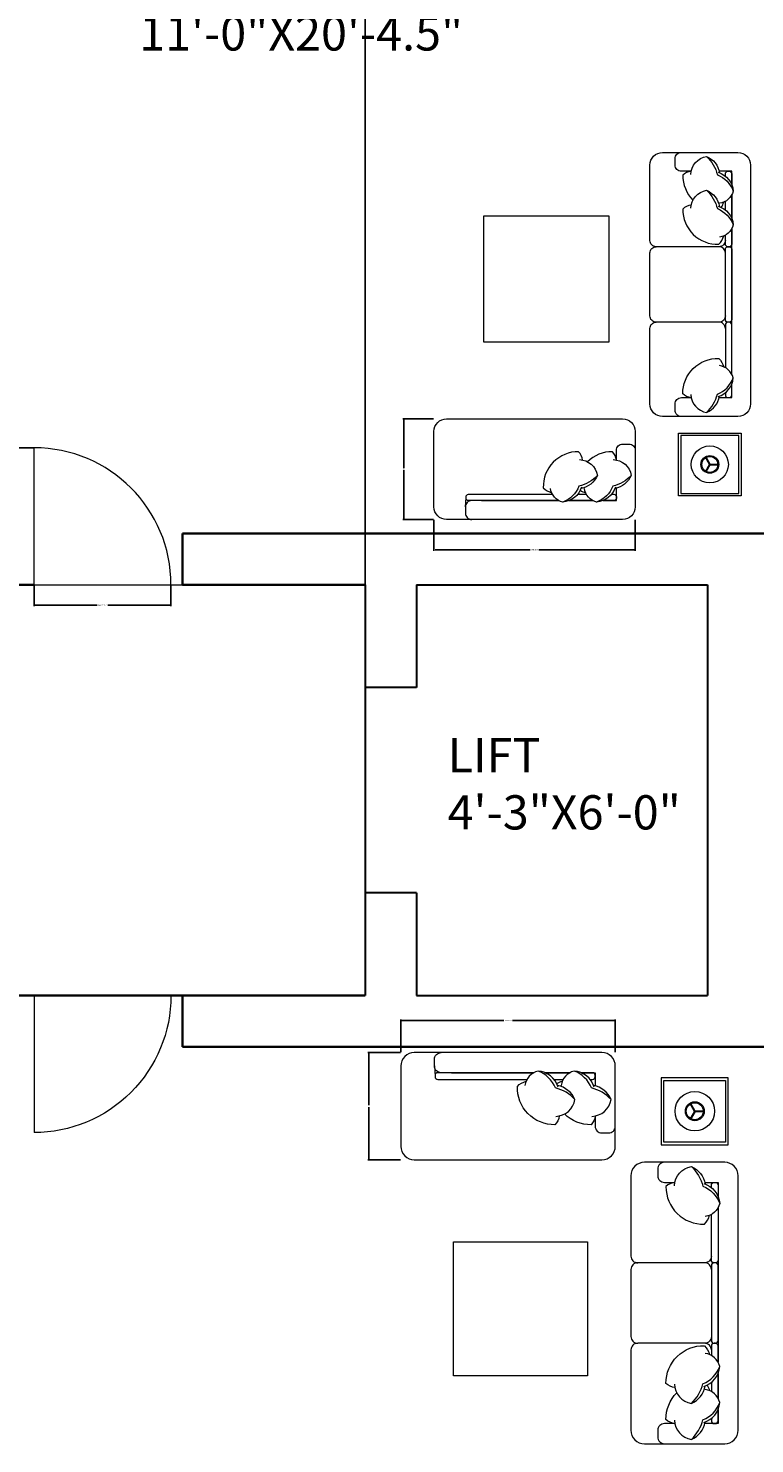
# Model space of a CAD drawing. Units: inches. Extents: x -59 to 444, y -680 to 63.
# Tile 6 of 9: x 132 to 260, y -423 to -175. Entities that reach past the tile are written whole.
import ezdxf

# ---------------------------------------------------------------- set-up
doc = ezdxf.new("R2010")
doc.units = ezdxf.units.IN
doc.header["$MEASUREMENT"] = 0
for name, color, linetype, lineweight in [('A-ANNO-DIMS', 2, 'Continuous', 18), ('A-AREA-IDEN', 7, 'Continuous', 18), ('A-DOOR', 3, 'Continuous', 18), ('A-FLOR-EVTR', 7, 'Continuous', 30), ('A-FURN', 8, 'Continuous', 13), ('A-WALL', 7, 'Continuous', 35)]:
    doc.layers.add(name, color=color, linetype=linetype, lineweight=lineweight)
doc.styles.get("Standard").update_dxf_attribs({"font": 'arial.ttf'})
doc.dimstyles.get("Standard").update_dxf_attribs({"dimtxt": 0.18, "dimasz": 0.18, "dimexe": 0.18, "dimexo": 0.0625, "dimgap": 0.09, "dimtad": 0, "dimtih": 1, "dimtoh": 1, "dimdec": 0, "dimzin": 0, "dimdsep": 46, "dimlunit": 3, "dimtxsty": 'Standard', "dimcen": 0.09, "dimadec": 0, "dimazin": 0, "dimtfac": 1, "dimtdec": 0, "dimtofl": 0, "dimtmove": 0, "dimatfit": 3, "dimfxl": 1, "dimtolj": 1, "dimtzin": 0, "dimarcsym": 0})

# ---------------------------------------------------------------- blocks, each defined once
blk = doc.blocks.new('DAY BED1')
at = {"color": 0}
blk.add_line((0.3, 0.25), (0.225, 0.255), dxfattribs=at)
blk.add_lwpolyline([(-0.3, 0, -0.414214), (-0.4, 0.1), (-0.4, 0.1, 0.317837), (-0.4, 0.1, -0.414214), (-0.4, 0.1), (-0.4, 0.1, 1.186185), (-0.4, 0.1, -0.414214), (-0.4, 0.1), (-0.4, 1.5, -0.414214), (-0.3, 1.6), (0.3, 1.6, -0.414214), (0.4, 1.5), (0.4, 0.1, -0.414214), (0.3, 0)], format="xyb", close=True, dxfattribs=at)
for points in [[(-0.073, 1.45), (-0.15, 1.45, -0.414214), (-0.2, 1.5), (-0.2, 1.55, -0.414214), (-0.15, 1.6)], [(-0.076, 1.425, -0.356772), (0.05, 1.568, -0.249542), (0.154, 1.438, 9.61688)], [(0.05, 1.568, -0.14773), (0.136, 1.422, -0.213343), (0.262, 1.293, -0.178662)], [(-0.073, 1.45, 0.165541), (-0.139, 1.419, 0.200231), (-0.058, 1.221, 0.121523)], [(0.143, 1.442, -0.306663), (0.262, 1.293, -0.30633), (0.154, 1.196, 0.872847)], [(0.25, 1.345), (0.25, 1.45), (0.152, 1.45, -0.414214)], [(0.2, 1.412), (0.2, 1.43, -0.414214), (0.22, 1.45), (0.23, 1.45, -0.414214), (0.25, 1.43)], [(0.25, 1.43), (0.25, 1.345, -0.414214)], [(-0.076, 1.156, -0.356772), (0.05, 1.299, -0.249542), (0.154, 1.169, 9.61688)], [(0.05, 1.299, -0.14773), (0.136, 1.153, -0.213343), (0.262, 1.024, -0.178662)], [(-0.073, 1.181, 0.165541), (-0.139, 1.15, 0.425989), (0.148, 0.869, 0.121523), (0.187, 0.936, -7.115464)], [(0.143, 1.173, -0.306663), (0.262, 1.024, -0.30633), (0.154, 0.926, 0.872847)], [(0.168, 1.163, 0.071865), (0.187, 1.205, -7.115464)], [(0.2, 1.142), (0.2, 1.211, -0.414214)], [(0.25, 1.262), (0.25, 1.075, -0.414214)], [(0.25, 0.992), (0.25, 0.275, -0.414214), (0.23, 0.255), (0.22, 0.255, -0.414214), (0.2, 0.275), (0.2, 0.942, -0.414214)], [(0.25, 0.377), (0.25, 0.3, 0.414214), (0.3, 0.25), (0.35, 0.25, 0.414214), (0.4, 0.3)]]:
    blk.add_lwpolyline(points, format="xyb", dxfattribs=at)
for points in [[(0.25, 1.075), (0.25, 1.262)], [(0.25, 0.377), (0.25, 0.992)]]:
    blk.add_lwpolyline(points, dxfattribs=at)
blk = doc.blocks.new('DOOR-SWING-24')
blk.add_line((24, 0), (0, 0))
blk.add_arc((24, 0), 24, 90, 180)
blk = doc.blocks.new('*D16')
at = {"layer": 'A-ANNO-DIMS', "color": 0, "lineweight": -2, "transparency": 16777216}
for p, q in [((133.23, -272.5), (133.23, -276.22)), ((157.23, -272.5), (157.23, -276.22)), ((133.41, -276.04), (144.29, -276.04)), ((157.05, -276.04), (146.17, -276.04))]:
    blk.add_line(p, q, dxfattribs=at)
at = {"layer": 'A-ANNO-DIMS', "color": 0, "transparency": 16777216}
for points in [[(133.41, -276.01), (133.41, -276.07), (133.23, -276.04)], [(157.05, -276.01), (157.05, -276.07), (157.23, -276.04)]]:
    blk.add_solid(points, dxfattribs=at)
at = {"layer": 'Defpoints', "color": 0, "transparency": 16777216}
for p in [(133.23, -272.44), (157.23, -272.44), (157.23, -276.04)]:
    blk.add_point(p, dxfattribs=at)
at = {"layer": 'A-ANNO-DIMS', "color": 0, "transparency": 16777216, "insert": (145.23, -276.04), "char_height": 0.18, "attachment_point": 5}
blk.add_mtext('\\A1;DOOR 24 TYP.', dxfattribs=at)
blk = doc.blocks.new('*D17')
at = {"layer": 'A-ANNO-DIMS', "color": 0, "lineweight": -2, "transparency": 16777216}
for p, q in [((133.17, -248.44), (129.45, -248.44)), ((129.63, -248.62), (129.63, -260.25)), ((129.63, -272.26), (129.63, -260.62)), ((133.17, -272.44), (129.45, -272.44))]:
    blk.add_line(p, q, dxfattribs=at)
at = {"layer": 'A-ANNO-DIMS', "color": 0, "transparency": 16777216}
for points in [[(129.6, -248.62), (129.66, -248.62), (129.63, -248.44)], [(129.6, -272.26), (129.66, -272.26), (129.63, -272.44)]]:
    blk.add_solid(points, dxfattribs=at)
at = {"layer": 'Defpoints', "color": 0, "transparency": 16777216}
for p in [(133.23, -248.44), (129.63, -272.44), (133.23, -272.44)]:
    blk.add_point(p, dxfattribs=at)
at = {"layer": 'A-ANNO-DIMS', "color": 0, "transparency": 16777216, "insert": (129.63, -260.44), "char_height": 0.18, "attachment_point": 5}
blk.add_mtext('\\A1;24 TYP.', dxfattribs=at)
blk = doc.blocks.new('*D42')
at = {"layer": 'A-ANNO-DIMS', "color": 0, "lineweight": -2, "transparency": 16777216}
for p, q in [((203.31, -261.07), (203.31, -266.48)), ((238.57, -261.07), (238.57, -266.48)), ((203.49, -266.3), (220.17, -266.3)), ((238.39, -266.3), (221.7, -266.3))]:
    blk.add_line(p, q, dxfattribs=at)
at = {"layer": 'A-ANNO-DIMS', "color": 0, "transparency": 16777216}
for points in [[(203.49, -266.27), (203.49, -266.33), (203.31, -266.3)], [(238.39, -266.27), (238.39, -266.33), (238.57, -266.3)]]:
    blk.add_solid(points, dxfattribs=at)
at = {"layer": 'Defpoints', "color": 0, "transparency": 16777216}
for p in [(203.31, -261.01), (238.57, -261.01), (238.57, -266.3)]:
    blk.add_point(p, dxfattribs=at)
at = {"layer": 'A-ANNO-DIMS', "color": 0, "transparency": 16777216, "insert": (220.94, -266.3), "char_height": 0.18, "attachment_point": 5}
blk.add_mtext('\\A1;DAYBED 35', dxfattribs=at)
blk = doc.blocks.new('*D43')
at = {"layer": 'A-ANNO-DIMS', "color": 0, "lineweight": -2, "transparency": 16777216}
for p, q in [((203.25, -243.38), (197.84, -243.38)), ((198.02, -243.56), (198.02, -252.01)), ((198.02, -260.83), (198.02, -252.38)), ((203.25, -261.01), (197.84, -261.01))]:
    blk.add_line(p, q, dxfattribs=at)
at = {"layer": 'A-ANNO-DIMS', "color": 0, "transparency": 16777216}
for points in [[(197.99, -243.56), (198.05, -243.56), (198.02, -243.38)], [(197.99, -260.83), (198.05, -260.83), (198.02, -261.01)]]:
    blk.add_solid(points, dxfattribs=at)
at = {"layer": 'Defpoints', "color": 0, "transparency": 16777216}
for p in [(203.31, -243.38), (198.02, -261.01), (203.31, -261.01)]:
    blk.add_point(p, dxfattribs=at)
at = {"layer": 'A-ANNO-DIMS', "color": 0, "transparency": 16777216, "insert": (198.02, -252.19), "char_height": 0.18, "attachment_point": 5}
blk.add_mtext('\\A1;18', dxfattribs=at)
blk = doc.blocks.new('*D44')
at = {"layer": 'A-ANNO-DIMS', "color": 0, "lineweight": -2, "transparency": 16777216}
for p, q in [((197.51, -354.37), (197.51, -348.62)), ((197.69, -348.8), (215.53, -348.8)), ((234.9, -348.8), (217.06, -348.8)), ((235.08, -354.37), (235.08, -348.62))]:
    blk.add_line(p, q, dxfattribs=at)
at = {"layer": 'A-ANNO-DIMS', "color": 0, "transparency": 16777216}
for points in [[(197.69, -348.77), (197.69, -348.83), (197.51, -348.8)], [(234.9, -348.77), (234.9, -348.83), (235.08, -348.8)]]:
    blk.add_solid(points, dxfattribs=at)
at = {"layer": 'Defpoints', "color": 0, "transparency": 16777216}
for p in [(235.08, -348.8), (197.51, -354.43), (235.08, -354.43)]:
    blk.add_point(p, dxfattribs=at)
at = {"layer": 'A-ANNO-DIMS', "color": 0, "transparency": 16777216, "insert": (216.29, -348.8), "char_height": 0.18, "attachment_point": 5}
blk.add_mtext('\\A1;DAYBED 38', dxfattribs=at)
blk = doc.blocks.new('*D45')
at = {"layer": 'A-ANNO-DIMS', "color": 0, "lineweight": -2, "transparency": 16777216}
for p, q in [((197.45, -354.43), (191.7, -354.43)), ((191.88, -354.61), (191.88, -363.64)), ((191.88, -373.03), (191.88, -364)), ((197.45, -373.21), (191.7, -373.21))]:
    blk.add_line(p, q, dxfattribs=at)
at = {"layer": 'A-ANNO-DIMS', "color": 0, "transparency": 16777216}
for points in [[(191.85, -354.61), (191.91, -354.61), (191.88, -354.43)], [(191.85, -373.03), (191.91, -373.03), (191.88, -373.21)]]:
    blk.add_solid(points, dxfattribs=at)
at = {"layer": 'Defpoints', "color": 0, "transparency": 16777216}
for p in [(191.88, -354.43), (197.51, -354.43), (197.51, -373.21)]:
    blk.add_point(p, dxfattribs=at)
at = {"layer": 'A-ANNO-DIMS', "color": 0, "transparency": 16777216, "insert": (191.88, -363.82), "char_height": 0.18, "attachment_point": 5}
blk.add_mtext('\\A1;19', dxfattribs=at)
blk = doc.blocks.new('*D56')
at = {"layer": 'A-ANNO-DIMS', "color": 0, "lineweight": -2, "transparency": 16777216}
for p, q in [((126.73, -344.37), (126.73, 62.74)), ((126.91, 62.56), (158.65, 62.56)), ((191.05, 62.56), (159.3, 62.56)), ((191.23, -344.37), (191.23, 62.74))]:
    blk.add_line(p, q, dxfattribs=at)
at = {"layer": 'A-ANNO-DIMS', "color": 0, "transparency": 16777216}
for points in [[(126.91, 62.59), (126.91, 62.53), (126.73, 62.56)], [(191.05, 62.59), (191.05, 62.53), (191.23, 62.56)]]:
    blk.add_solid(points, dxfattribs=at)
at = {"layer": 'Defpoints', "color": 0, "transparency": 16777216}
for p in [(191.23, 62.56), (126.73, -344.44), (191.23, -344.44)]:
    blk.add_point(p, dxfattribs=at)
at = {"layer": 'A-ANNO-DIMS', "color": 0, "transparency": 16777216, "insert": (158.98, 62.56), "char_height": 0.18, "attachment_point": 5}
blk.add_mtext('\\A1;64.5', dxfattribs=at)

msp = doc.modelspace()

# ---------------------------------------------------------------- linework, layer by layer
at = {"layer": 'A-DOOR'}
for p, q in [((133.23, -272.44), (157.23, -272.44)), ((157.23, -272.44), (159.23, -272.44))]:
    msp.add_line(p, q, dxfattribs=at)
at = {"layer": 'A-FLOR-EVTR'}
for p, q in [((191.23, -272.44), (191.23, -344.44)), ((200.23, -272.44), (200.23, -290.44)), ((200.23, -272.44), (251.23, -272.44)), ((251.23, -272.44), (251.23, -344.44)), ((200.23, -290.44), (191.23, -290.44)), ((200.23, -326.44), (191.23, -326.44)), ((200.23, -326.44), (200.23, -344.44)), ((200.23, -344.44), (251.23, -344.44))]:
    msp.add_line(p, q, dxfattribs=at)
at = {"layer": 'A-FURN'}
for p, q in [((251.58, -251.4), (250.8, -250.05)), ((251.7, -251.33), (250.92, -249.98)), ((251.58, -251.33), (250.8, -252.68)), ((251.7, -251.4), (250.92, -252.74)), ((251.64, -251.3), (253.19, -251.3)), ((251.64, -251.43), (253.19, -251.43)), ((248.94, -364.74), (248.12, -363.31)), ((249.07, -364.67), (248.24, -363.24)), ((248.94, -364.67), (248.12, -366.1)), ((249.07, -364.74), (248.24, -366.18)), ((249.01, -364.63), (250.66, -364.63)), ((249.01, -364.78), (250.66, -364.78))]:
    msp.add_line(p, q, dxfattribs=at)
at = {"layer": 'A-FURN', "ltscale": 0.03}
for points in [[(243.35, -242.96, -0.414214), (241.14, -240.76), (241.14, -227.54, -0.414214), (242.24, -226.43, -0.414214), (241.14, -225.33), (241.14, -214.31, -0.414214), (242.24, -213.21, -0.414214), (241.14, -212.11), (241.14, -198.89, -0.414214), (243.35, -196.69), (256.57, -196.69, -0.414214), (258.77, -198.89), (258.77, -240.76, -0.414214), (256.57, -242.96)], [(240.17, -373.66, 0.414214), (237.82, -376.01), (237.82, -390.1, 0.414214), (239, -391.27, 0.414214), (237.82, -392.44), (237.82, -404.18, 0.414214), (239, -405.36, 0.414214), (237.82, -406.53), (237.82, -420.62, 0.414214), (240.17, -422.97), (254.26, -422.97, 0.414214), (256.61, -420.62), (256.61, -376.01, 0.414214), (254.26, -373.66)]]:
    msp.add_lwpolyline(points, format="xyb", close=True, dxfattribs=at)
at = {"layer": 'A-FURN'}
for points in [[(248.36, -199.99), (246.65, -199.99, -0.414214), (245.55, -198.89), (245.55, -197.79, -0.414214), (246.65, -196.69)], [(248.29, -200.54, -0.356772), (251.07, -197.39, -0.249542), (253.36, -200.25, 9.61688)], [(251.07, -197.39, -0.14773), (252.96, -200.61, -0.213343), (255.74, -203.45, -0.178662)], [(248.36, -199.99, 0.165541), (246.9, -200.67, 0.200231), (248.68, -205.04, 0.121523)], [(253.11, -200.16, -0.306663), (255.74, -203.45, -0.30633), (253.34, -205.6, 0.872847)], [(255.47, -202.31), (255.47, -199.99), (253.3, -199.99, -0.414214)], [(254.36, -200.83), (254.36, -200.43, -0.414214), (254.8, -199.99), (255.02, -199.99, -0.414214), (255.47, -200.43)], [(255.47, -200.43), (255.47, -202.31, -0.414214)], [(248.29, -206.48, -0.356772), (251.07, -203.32, -0.249542), (253.36, -206.18, 9.61688)], [(251.07, -203.32, -0.14773), (252.96, -206.54, -0.213343), (255.74, -209.38, -0.178662)], [(253.65, -206.31, 0.071865), (254.08, -205.39, -7.115464)], [(254.36, -206.77), (254.36, -205.25, -0.414214)], [(255.47, -204.14), (255.47, -208.24, -0.414214)], [(248.36, -205.92, 0.165541), (246.9, -206.61, 0.425989), (253.21, -212.79, 0.121523), (254.08, -211.32, -7.115464)], [(253.11, -206.1, -0.306663), (255.74, -209.38, -0.30633), (253.34, -211.53, 0.872847)], [(255.47, -210.08), (255.47, -212.77, -0.414214), (255.02, -213.21), (254.8, -213.21, -0.414214), (254.36, -212.77), (254.36, -211.19, -0.414214)], [(254.36, -212.11, -0.414214), (253.26, -213.21), (242.24, -213.21, -0.414214)], [(254.36, -214.31, 0.414214), (253.26, -213.21)], [(254.36, -225.33, -0.414214), (253.26, -226.43)], [(254.36, -227.54, 0.414214), (253.26, -226.43), (242.24, -226.43, 0.414214)], [(255.47, -235.5), (255.47, -226.87, 0.414214), (255.02, -226.43), (254.8, -226.43, 0.414214), (254.36, -226.87), (254.36, -234.4, 0.414214)], [(248.36, -239.66, -0.165541), (246.9, -238.98, -0.425989), (253.21, -232.79, -0.121523), (254.08, -234.26, 7.115464)], [(253.11, -239.48, 0.306663), (255.74, -236.2, 0.30633), (253.34, -234.05, -0.872847)], [(251.07, -242.26, 0.14773), (252.96, -239.04, 0.213343), (255.74, -236.2, 0.178662)], [(255.47, -239.21), (255.47, -237.34, 0.414214)], [(246.65, -242.96, -0.414214), (245.55, -241.86), (245.55, -240.76, -0.414214), (246.65, -239.66), (248.36, -239.66)], [(248.29, -239.1, 0.356772), (251.07, -242.26, 0.249542), (253.36, -239.4, -9.61688)], [(254.36, -238.81), (254.36, -239.21, 0.414214), (254.8, -239.66), (255.02, -239.66, 0.414214), (255.47, -239.21)], [(243.69, -373.66, 0.414214), (242.52, -374.83), (242.52, -376.01, 0.414214), (243.69, -377.18), (245.51, -377.18)], [(245.44, -377.77, -0.356772), (248.4, -374.41, -0.249542), (250.84, -377.45, 9.61688)], [(248.4, -374.41, -0.14773), (250.42, -377.84, -0.213343), (253.38, -380.87, -0.178662)], [(245.51, -377.18, 0.165541), (243.96, -377.91, 0.425989), (250.69, -384.5, 0.121523), (251.61, -382.93, -7.115464)], [(250.58, -377.36, -0.306663), (253.38, -380.87, -0.30633), (250.82, -383.15, 0.872847)], [(251.91, -378.08), (251.91, -377.65, -0.414214), (252.38, -377.18), (252.61, -377.18, -0.414214), (253.08, -377.65)], [(253.08, -377.65), (253.08, -379.65, -0.414214)], [(253.08, -381.6), (253.08, -390.8, -0.414214), (252.61, -391.27), (252.38, -391.27, -0.414214), (251.91, -390.8), (251.91, -382.79, -0.414214)], [(251.91, -390.1, -0.414214), (250.74, -391.27), (239, -391.27, -0.414214)], [(251.91, -392.44, 0.414214), (250.74, -391.27)], [(251.91, -404.18, -0.414214), (250.74, -405.36)], [(251.91, -406.53, 0.414214), (250.74, -405.36), (239, -405.36, 0.414214)], [(245.51, -413.12, -0.165541), (243.96, -412.4, -0.425989), (250.69, -405.8, -0.121523), (251.61, -407.37, 7.115464)], [(253.08, -408.7), (253.08, -405.83, 0.414214), (252.61, -405.36), (252.38, -405.36, 0.414214), (251.91, -405.83), (251.91, -407.52, 0.414214)], [(250.58, -412.94, 0.306663), (253.38, -409.44, 0.30633), (250.82, -407.15, -0.872847)], [(248.4, -415.9, 0.14773), (250.42, -412.46, 0.213343), (253.38, -409.44, 0.178662)], [(253.08, -415.02), (253.08, -410.65, 0.414214)], [(245.51, -419.45, -0.165541), (243.96, -418.72, -0.200231), (245.85, -414.06, -0.121523)], [(245.44, -412.53, 0.356772), (248.4, -415.9, 0.249542), (250.84, -412.85, -9.61688)], [(250.58, -419.26, 0.306663), (253.38, -415.76, 0.30633), (250.82, -413.47, -0.872847)], [(251.15, -412.71, -0.071865), (251.61, -413.69, 7.115464)], [(251.91, -412.22), (251.91, -413.84, 0.414214)], [(248.4, -422.22, 0.14773), (250.42, -418.79, 0.213343), (253.38, -415.76, 0.178662)], [(245.44, -418.86, 0.356772), (248.4, -422.22, 0.249542), (250.84, -419.17, -9.61688)], [(253.08, -416.97), (253.08, -419.44), (250.78, -419.44, 0.414214)], [(251.91, -418.55), (251.91, -418.97, 0.414214), (252.38, -419.44), (252.61, -419.44, 0.414214), (253.08, -418.97)], [(253.08, -418.97), (253.08, -416.97, 0.414214)], [(245.51, -419.44), (243.69, -419.44, 0.414214), (242.52, -420.62), (242.52, -421.79, 0.414214), (243.69, -422.97)]]:
    msp.add_lwpolyline(points, format="xyb", dxfattribs=at)
for points in [[(255.47, -208.24), (255.47, -204.14)], [(255.47, -235.5), (255.47, -210.08)], [(253.3, -239.66), (255.47, -239.66), (255.47, -237.34)], [(250.78, -377.18), (253.08, -377.18), (253.08, -379.65)], [(253.08, -381.6), (253.08, -408.7)], [(253.08, -410.65), (253.08, -415.02)]]:
    msp.add_lwpolyline(points, dxfattribs=at)
at = {"layer": 'A-FURN', "ltscale": 0.03}
for points in [[(211.97, -207.84), (211.97, -229.88), (234.01, -229.88), (234.01, -207.84)], [(246.13, -256.87), (246.13, -245.86), (257.15, -245.86), (257.15, -256.87)], [(243.14, -358.84), (243.14, -370.58), (254.88, -370.58), (254.88, -358.84)], [(206.75, -411.08), (206.75, -387.6), (230.22, -387.6), (230.22, -411.08)]]:
    msp.add_lwpolyline(points, close=True, dxfattribs=at)
at = {"layer": 'A-FURN'}
for points in [[(255.47, -213.65), (255.47, -225.99, -0.414214), (255.02, -226.43), (254.8, -226.43, -0.414214), (254.36, -225.99), (254.36, -213.65, -0.414214), (254.8, -213.21), (255.02, -213.21, -0.414214)], [(253.08, -404.89), (253.08, -391.74, 0.414214), (252.61, -391.27), (252.38, -391.27, 0.414214), (251.91, -391.74), (251.91, -404.89, 0.414214), (252.38, -405.36), (252.61, -405.36, 0.414214)]]:
    msp.add_lwpolyline(points, format="xyb", close=True, dxfattribs=at)
for points in [[(246.57, -246.3), (246.57, -256.43), (256.71, -256.43), (256.71, -246.3)], [(243.61, -370.11), (243.61, -359.31), (254.41, -359.31), (254.41, -370.11)]]:
    msp.add_lwpolyline(points, close=True, dxfattribs=at)
for centre, radius in [((251.64, -251.36), 3.25), ((251.64, -251.36), 1.56), ((251.64, -251.36), 1.39), ((249.01, -364.71), 3.46), ((249.01, -364.71), 1.66), ((249.01, -364.71), 1.49)]:
    msp.add_circle(centre, radius, dxfattribs=at)
at = {"layer": 'A-WALL'}
for p, q in [((159.23, -272.44), (159.23, -263.44)), ((159.23, -263.44), (263.23, -263.44)), ((10.73, -272.44), (133.23, -272.44)), ((159.23, -272.44), (191.23, -272.44)), ((10.73, -344.44), (191.23, -344.44)), ((159.23, -344.44), (159.23, -353.44)), ((159.23, -353.44), (263.23, -353.44))]:
    msp.add_line(p, q, dxfattribs=at)

# ---------------------------------------------------------------- block references
at = {"layer": 'A-DOOR', "rotation": 270.0000000000001}
msp.add_blockref('DOOR-SWING-24', (133.23, -248.44), dxfattribs=at)
at = {"layer": 'A-DOOR', "extrusion": (0, 0, -1), "zscale": -1, "rotation": 89.99999999999999}
msp.add_blockref('DOOR-SWING-24', (-133.23, -368.44), dxfattribs=at)
at = {"layer": 'A-FURN', "ltscale": 0.03, "rotation": 270}
for p, xscale, yscale, zscale in [((203.31, -252.19), 22.03586383601939, 22.03586383601939, 22.03586383601939), ((197.51, -363.82), -23.47931942090405, 23.47931942090405, 23.47931942090405)]:
    msp.add_blockref('DAY BED1', p, dxfattribs=dict(at, xscale=xscale, yscale=yscale, zscale=zscale))

# ---------------------------------------------------------------- texts
at = {"layer": 'A-AREA-IDEN', "char_height": 6, "attachment_point": 1}
for s, insert in [('LIVING\\P11\'-0"X20\'-4.5"', (151.66, -162.83)), ('LIFT\\P4\'-3"X6\'-0"', (205.7, -299.33))]:
    msp.add_mtext(s, dxfattribs=dict(at, insert=insert))

# ---------------------------------------------------------------- dimensions: what is measured, and where the dimension line sits
at = {"layer": 'A-ANNO-DIMS'}
dim = msp.add_linear_dim(base=(191.23, 62.56), p1=(126.73, -344.44), p2=(191.23, -344.44), dimstyle='Standard', override={"dimdec": 1, "dimlfac": 1, "dimrnd": 0, "dimzin": 0, "dimdsep": 46, "dimlunit": 2}, dxfattribs=at)
dim.commit()
dim.dimension.update_dxf_attribs({"geometry": '*D56', "text_midpoint": (158.98, 62.56)})
for base, p1, p2, angle, picture, middle in [((198.02, -261.01), (203.31, -243.38), (203.31, -261.01), 270, '*D43', (198.02, -252.19)), ((191.88, -354.43), (197.51, -373.21), (197.51, -354.43), 90, '*D45', (191.88, -363.82))]:
    dim = msp.add_linear_dim(base=base, p1=p1, p2=p2, angle=angle, dimstyle='Standard', override={"dimdec": 0, "dimlfac": 1, "dimrnd": 0, "dimzin": 0, "dimdsep": 46, "dimlunit": 2}, dxfattribs=at)
    dim.commit()
    dim.dimension.update_dxf_attribs({"geometry": picture, "text_midpoint": middle})
for base, p1, p2, angle, text, picture, middle in [((129.63, -272.44), (133.23, -248.44), (133.23, -272.44), 270, '<> TYP.', '*D17', (129.63, -260.44)), ((157.23, -276.04), (133.23, -272.44), (157.23, -272.44), 0, 'DOOR <> TYP.', '*D16', (145.23, -276.04))]:
    dim = msp.add_linear_dim(base=base, p1=p1, p2=p2, angle=angle, text=text, dimstyle='Standard', override={"dimdec": 0, "dimlfac": 1, "dimrnd": 0, "dimzin": 0, "dimdsep": 46, "dimlunit": 2}, dxfattribs=at)
    dim.commit()
    dim.dimension.update_dxf_attribs({"geometry": picture, "text_midpoint": middle})
for base, p1, p2, picture, middle in [((238.57, -266.3), (203.31, -261.01), (238.57, -261.01), '*D42', (220.94, -266.3)), ((235.08, -348.8), (197.51, -354.43), (235.08, -354.43), '*D44', (216.29, -348.8))]:
    dim = msp.add_linear_dim(base=base, p1=p1, p2=p2, text='DAYBED <>', dimstyle='Standard', override={"dimdec": 0, "dimlfac": 1, "dimrnd": 0, "dimzin": 0, "dimdsep": 46, "dimlunit": 2}, dxfattribs=at)
    dim.commit()
    dim.dimension.update_dxf_attribs({"geometry": picture, "text_midpoint": middle})

doc.saveas('drawing.dxf')
